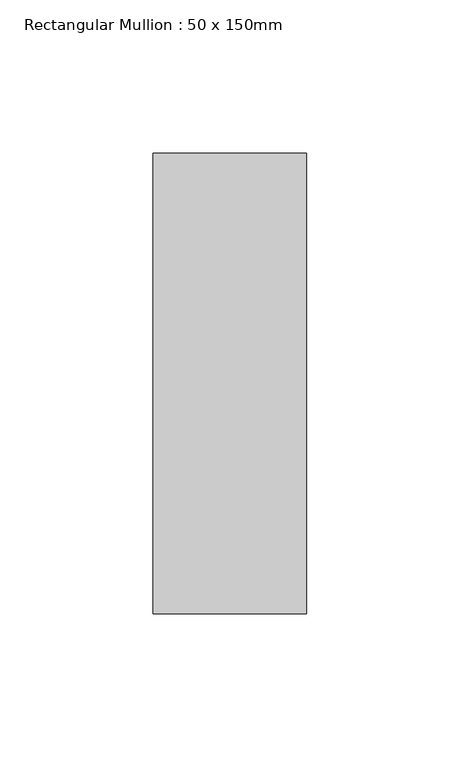
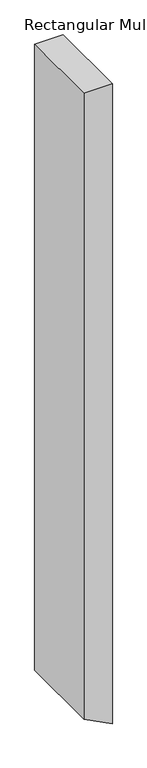
"""IFC4 building model written with IfcOpenShell, lengths in millimetres: member geometry, Rectangular Mullion : 50 x 150mm."""

from ifc_helpers import new_model, si_unit, frame, origin, place, context, project, spatial, polyline, outline, extrude, source, transform, mapped, element, save


def rectangular_mullion_50_x_150mm_0e9b4e8c(model_context):
    return source(origin(), model_context, "Body", "SweptSolid", [
        extrude(outline(polyline([(0.0, 0.0), (0.0, -50.0), (-1164.2268715, -50.0), (-1190.255224, 0.0), (0.0, 0.0)])), frame((0.0, -75.0, 0.0), z_axis=(0.0, 1.0, 0.0), x_axis=(0.0, 0.0, 1.0)), (0.0, 0.0, 1.0), 150.0),
    ])


if __name__ == "__main__":
    model = new_model("IFC4")
    model_context = context("Model", 3, world=origin())
    ifc_project = project(units=[si_unit("LENGTHUNIT", "METRE", prefix="MILLI")], contexts=[model_context])
    site = spatial("IfcSite", under=ifc_project)
    building = spatial("IfcBuilding", under=site)
    placement = place(None, origin())
    rectangular_mullion_50_x_150mm_shape = rectangular_mullion_50_x_150mm_0e9b4e8c(model_context)
    element("IfcMember", 1, ObjectType="Rectangular Mullion : 50 x 150mm", at=placement, inside=building, context=model_context, shape_type="MappedRepresentation", body=[
        mapped(rectangular_mullion_50_x_150mm_shape, transform((0.0, 0.0, 0.0), x_axis=(1.0, 0.0, 0.0), y_axis=(0.0, 1.0, 0.0), z_axis=(0.0, 0.0, 1.0))),
    ])
    save(model, "model.ifc")

# Revit data of these elements
# Type "Rectangular Mullion : 50 x 150mm"
#   built-in parameter 1007304 = 0.492126 (stored number, unit not read)
#   built-in parameter 1007301 = 0.082021 (stored number, unit not read)
#   built-in parameter 1007300 = 0.082021 (stored number, unit not read)
# Element 1 (IfcMember, "Rectangular Mullion : 50 x 150mm")
#   Materials on its faces: "Aluminium"
# Materials
#   "Aluminium": class "Metal", colour RGB 247 247 247, transparency 0, Description = "Aluminium 6061", Cost = 0
